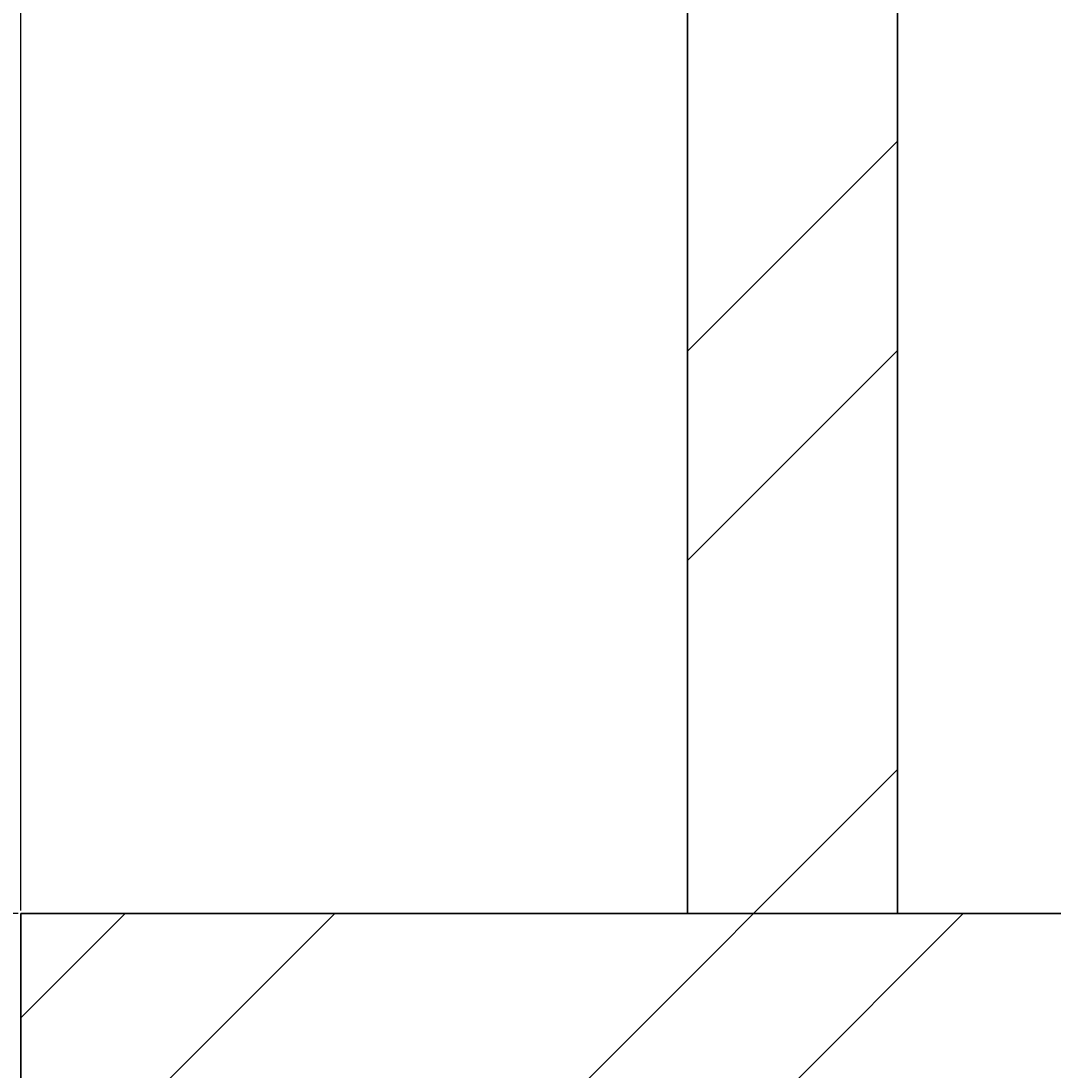
# Model space of a CAD drawing. Units: inches. Extents: x 1962 to 2771, y 1245 to 2660.
# Tile 38 of 114: x 2072.02 to 2094.14, y 2030.47 to 2052.97. Entities that reach past the tile are written whole.
import ezdxf

# ---------------------------------------------------------------- set-up
doc = ezdxf.new("R2010")
doc.units = ezdxf.units.IN
for name, color, linetype, lineweight in [('A-ANNO-DIMS', 2, 'Continuous', 18), ('A-WALL', 7, 'Continuous', 35), ('A-WALL-PATT', 252, 'Continuous', 13)]:
    doc.layers.add(name, color=color, linetype=linetype, lineweight=lineweight)
doc.styles.get("Standard").update_dxf_attribs({"font": 'arial.ttf'})
doc.dimstyles.get("Standard").update_dxf_attribs({"dimtxt": 0.18, "dimasz": 0.18, "dimexe": 0.18, "dimexo": 0.0625, "dimgap": 0.09, "dimtad": 0, "dimtih": 1, "dimtoh": 1, "dimdec": 4, "dimzin": 0, "dimdsep": 46, "dimtxsty": 'Standard', "dimcen": 0.09, "dimadec": 0, "dimazin": 0, "dimtfac": 1, "dimtdec": 4, "dimtofl": 0, "dimtmove": 0, "dimatfit": 3, "dimfxl": 1, "dimtolj": 1, "dimtzin": 0, "dimarcsym": 0})

# ---------------------------------------------------------------- blocks, each defined once
blk = doc.blocks.new('*D40')
at = {"layer": 'A-ANNO-DIMS', "color": 0, "lineweight": -2, "transparency": 16777216}
for p, q in [((2072.02, 2033.906), (2072.02, 2583.474)), ((2660.807, 2524.406), (2660.807, 2583.474)), ((2072.2, 2583.294), (2366.02, 2583.294)), ((2660.627, 2583.294), (2366.808, 2583.294))]:
    blk.add_line(p, q, dxfattribs=at)
at = {"layer": 'A-ANNO-DIMS', "color": 0, "transparency": 16777216}
for points in [[(2072.2, 2583.324), (2072.2, 2583.264), (2072.02, 2583.294)], [(2660.627, 2583.324), (2660.627, 2583.264), (2660.807, 2583.294)]]:
    blk.add_solid(points, dxfattribs=at)
at = {"layer": 'Defpoints', "color": 0, "transparency": 16777216}
for p in [(2660.807, 2583.294), (2660.807, 2524.344), (2072.02, 2033.844)]:
    blk.add_point(p, dxfattribs=at)
at = {"layer": 'A-ANNO-DIMS', "color": 0, "transparency": 16777216, "insert": (2366.414, 2583.294), "char_height": 0.18, "attachment_point": 5}
blk.add_mtext('\\A1;588.8', dxfattribs=at)
blk = doc.blocks.new('*D43')
at = {"layer": 'A-ANNO-DIMS', "color": 0, "lineweight": -2, "transparency": 16777216}
for p, q in [((2086.245, 2524.344), (2012.89, 2524.344)), ((2013.07, 2524.164), (2013.07, 2279.276)), ((2013.07, 2034.024), (2013.07, 2278.912)), ((2071.958, 2033.844), (2012.89, 2033.844))]:
    blk.add_line(p, q, dxfattribs=at)
at = {"layer": 'A-ANNO-DIMS', "color": 0, "transparency": 16777216}
for points in [[(2013.04, 2524.164), (2013.1, 2524.164), (2013.07, 2524.344)], [(2013.04, 2034.024), (2013.1, 2034.024), (2013.07, 2033.844)]]:
    blk.add_solid(points, dxfattribs=at)
at = {"layer": 'Defpoints', "color": 0, "transparency": 16777216}
for p in [(2086.307, 2524.344), (2013.07, 2033.844), (2072.02, 2033.844)]:
    blk.add_point(p, dxfattribs=at)
at = {"layer": 'A-ANNO-DIMS', "color": 0, "transparency": 16777216, "insert": (2013.07, 2279.094), "char_height": 0.18, "attachment_point": 5}
blk.add_mtext('\\A1;490.5', dxfattribs=at)

msp = doc.modelspace()

# ---------------------------------------------------------------- hatches: boundary and pattern name
at = {"layer": 'A-WALL-PATT'}
h = msp.add_hatch(dxfattribs=at)
h.set_pattern_fill('ANSI32', color=256)
h.paths.add_polyline_path([(2090.8074, 2467.3437), (2141.6481, 2467.3437), (2141.6481, 2469.5937), (2141.6481, 2471.8437), (2086.3074, 2471.8437), (2086.3074, 2422.5333), (2090.8074, 2422.5333)])
h.paths.add_polyline_path([(2282.7664, 2471.8437), (2204.8982, 2471.8437), (2204.8982, 2467.3437), (2234.8074, 2467.3437), (2234.8074, 2311.3437), (2228.7492, 2311.3437), (2228.7492, 2306.8437), (2234.8074, 2306.8437), (2331.9227, 2306.8437), (2331.9227, 2309.0937), (2331.9227, 2311.3437), (2239.3074, 2311.3437), (2239.3074, 2467.3437), (2282.7664, 2467.3437), (2282.7664, 2469.5937)])
h.paths.add_polyline_path([(2471.4531, 2519.8437), (2552.011, 2519.8437), (2564.3996, 2519.8437), (2564.3996, 2511.1389), (2568.8996, 2511.1389), (2568.8996, 2524.3437), (2466.9531, 2524.3437), (2466.9531, 2471.8437), (2450.0749, 2471.8437), (2446.4672, 2471.8437), (2446.4672, 2467.3437), (2450.0749, 2467.3437), (2475.9988, 2467.3437), (2475.9988, 2469.5937), (2475.9988, 2471.8437), (2471.4531, 2471.8437)])
h.paths.add_polyline_path([(2575.2231, 2469.5937), (2575.2231, 2471.8437), (2568.8996, 2471.8437), (2568.8996, 2487.1389), (2564.3996, 2487.1389), (2564.3996, 2471.8437), (2556.511, 2471.8437), (2499.2904, 2471.8437), (2499.2904, 2467.3437), (2507.8074, 2467.3437), (2507.8074, 2311.3437), (2414.863, 2311.3437), (2414.863, 2306.8437), (2512.3074, 2306.8437), (2517.0114, 2306.8437), (2517.0114, 2309.0937), (2517.0114, 2311.3437), (2512.3074, 2311.3437), (2512.3074, 2467.3437), (2575.2231, 2467.3437)])
h.paths.add_polyline_path([(2660.8074, 2471.8437), (2600.9602, 2471.8437), (2600.9602, 2467.3437), (2656.3074, 2467.3437), (2656.3074, 2432.5704), (2660.8074, 2432.5704)])
h.paths.add_polyline_path([(2660.8074, 2372.5704), (2656.3074, 2372.5704), (2656.3074, 2311.3437), (2600.276, 2311.3437), (2600.276, 2309.0937), (2600.276, 2306.8437), (2656.3074, 2306.8437), (2656.3074, 2296.2593), (2660.8074, 2296.2593)])
h.paths.add_polyline_path([(2572.3074, 2306.8437), (2577.1385, 2306.8437), (2577.1385, 2311.3437), (2551.082, 2311.3437), (2551.082, 2306.8437), (2567.8074, 2306.8437), (2567.8074, 2258.8437), (2540.0574, 2258.8437), (2540.0574, 2256.5937), (2540.0574, 2254.3437), (2567.8074, 2254.3437), (2656.3074, 2254.3437), (2656.3074, 2236.9085), (2660.8074, 2236.9085), (2660.8074, 2272.2593), (2656.3074, 2272.2593), (2656.3074, 2258.8437), (2572.3074, 2258.8437)])
h.paths.add_polyline_path([(2512.3074, 2254.3437), (2518.8716, 2254.3437), (2518.8716, 2256.5937), (2518.8716, 2258.8437), (2507.8074, 2258.8437), (2507.8074, 2177.8437), (2567.8074, 2177.8437), (2567.8074, 2172.9628), (2572.3074, 2172.9628), (2572.3074, 2177.8437), (2656.3074, 2177.8437), (2656.3074, 2166.4846), (2660.8074, 2166.4846), (2660.8074, 2200.9085), (2656.3074, 2200.9085), (2656.3074, 2182.3437), (2512.3074, 2182.3437)])
h.paths.add_polyline_path([(2656.3074, 2129.8437), (2572.3074, 2129.8437), (2572.3074, 2150.3044), (2570.0574, 2150.3044), (2567.8074, 2150.3044), (2567.8074, 2129.8437), (2507.8074, 2129.8437), (2507.8074, 2116.3027), (2510.0574, 2116.3027), (2512.3074, 2116.3027), (2512.3074, 2125.3437), (2567.8074, 2125.3437), (2572.3074, 2125.3437), (2656.3074, 2125.3437)])
h.paths.add_polyline_path([(2090.8074, 2362.5333), (2086.3074, 2362.5333), (2086.3074, 2298.6242), (2090.8074, 2298.6242), (2090.8074, 2306.8437), (2174.8074, 2306.8437), (2174.8074, 2286.4178), (2179.3074, 2286.4178), (2179.3074, 2306.8437), (2192.8641, 2306.8437), (2192.8641, 2309.0937), (2192.8641, 2311.3437), (2090.8074, 2311.3437)])
h.paths.add_polyline_path([(2209.156, 2258.8437), (2179.3074, 2258.8437), (2179.3074, 2263.2236), (2177.0574, 2263.2236), (2174.8074, 2263.2236), (2174.8074, 2258.8437), (2090.8074, 2258.8437), (2090.8074, 2274.6242), (2086.3074, 2274.6242), (2086.3074, 2238.2967), (2088.5574, 2238.2967), (2090.8074, 2238.2967), (2090.8074, 2254.3437), (2209.156, 2254.3437)])
h.paths.add_polyline_path([(2090.8074, 2177.8437), (2234.8074, 2177.8437), (2234.8074, 2173.1428), (2239.3074, 2173.1428), (2239.3074, 2258.8437), (2230.8442, 2258.8437), (2230.8442, 2256.5937), (2230.8442, 2254.3437), (2234.8074, 2254.3437), (2234.8074, 2182.3437), (2090.8074, 2182.3437), (2090.8074, 2202.2967), (2086.3074, 2202.2967), (2086.3074, 2140.0389), (2090.8074, 2140.0389)])
h.paths.add_polyline_path([(2090.8074, 2080.0389), (2086.3074, 2080.0389), (2086.3074, 2033.8437), (2090.8074, 2033.8437)], flags=17)
h.paths.add_polyline_path([(2244.9405, 2033.8437), (2239.3074, 2033.8437), (2239.3074, 2142.0665), (2237.2592, 2142.0665), (2234.8074, 2142.0665), (2234.8074, 2033.8437), (2090.8074, 2033.8437), (2076.5204, 2033.8437), (2072.0204, 2033.8437), (2072.0204, 2000.4493), (2076.5204, 2000.4493), (2076.5204, 2029.3437), (2090.8074, 2029.3437), (2244.9405, 2029.3437), (2244.9405, 2031.5937)])
h.paths.add_polyline_path([(2234.8074, 1933.3437), (2076.5204, 1933.3437), (2076.5204, 1952.4493), (2074.2704, 1952.4493), (2072.0204, 1952.4493), (2072.0204, 1933.3437), (2072.0204, 1928.8437), (2234.8074, 1928.8437)])
h.paths.add_polyline_path([(2090.8074, 1928.8437), (2086.3074, 1928.8437), (2086.3074, 1906.5013), (2090.8074, 1906.5013)])
h.paths.add_polyline_path([(2090.8074, 1846.5013), (2086.3074, 1846.5013), (2086.3074, 1769.9917), (2088.5574, 1769.9917), (2090.8074, 1769.9917), (2090.8074, 1780.3437), (2234.8074, 1780.3437), (2234.8074, 1708.3437), (2230.3764, 1708.3437), (2230.3764, 1703.8437), (2239.3074, 1703.8437), (2239.3074, 1792.6669), (2237.0574, 1792.6669), (2234.8074, 1792.6669), (2234.8074, 1784.8437), (2090.8074, 1784.8437)])
h.paths.add_polyline_path([(2239.3074, 1928.8437), (2244.9405, 1928.8437), (2244.9405, 1931.0937), (2244.9405, 1933.3437), (2234.8074, 1933.3437), (2234.8074, 1928.8437), (2234.8074, 1825.5949), (2239.3074, 1825.5949)])
h.paths.add_polyline_path([(2148.0425, 1649.0937), (2148.0425, 1651.3437), (2090.8074, 1651.3437), (2090.8074, 1646.8437), (2148.0425, 1646.8437)], flags=0)
h.paths.add_polyline_path([(2207.5601, 1708.3437), (2090.8074, 1708.3437), (2090.8074, 1703.8437), (2174.8074, 1703.8437), (2174.8074, 1651.3437), (2170.4457, 1651.3437), (2170.4457, 1646.8437), (2195.9924, 1646.8437), (2195.9924, 1649.0937), (2195.9924, 1651.3437), (2179.3074, 1651.3437), (2179.3074, 1703.8437), (2207.5601, 1703.8437), (2207.5601, 1706.0937)])
h.paths.add_polyline_path([(2090.8074, 1733.9917), (2086.3074, 1733.9917), (2086.3074, 1696.1032), (2088.5574, 1696.1032), (2090.8074, 1696.1032)])
h.paths.add_polyline_path([(2090.8074, 1672.1032), (2086.3074, 1672.1032), (2086.3074, 1600.3335), (2090.8074, 1600.3335)])
h.paths.add_polyline_path([(2090.8074, 1540.3335), (2086.3074, 1540.3335), (2086.3074, 1486.3437), (2139.6766, 1486.3437), (2139.6766, 1490.8437), (2090.8074, 1490.8437)])
h.paths.add_polyline_path([(2302.3876, 1490.8437), (2239.3074, 1490.8437), (2239.3074, 1646.8437), (2335.9994, 1646.8437), (2335.9994, 1651.3437), (2229.884, 1651.3437), (2229.884, 1646.8437), (2234.8074, 1646.8437), (2234.8074, 1490.8437), (2202.7103, 1490.8437), (2202.7103, 1488.5937), (2202.7103, 1486.3437), (2275.0699, 1486.3437), (2275.0699, 1475.772), (2279.5699, 1475.772), (2279.5699, 1486.3437), (2302.3876, 1486.3437)])
h.paths.add_polyline_path([(2279.5699, 1451.772), (2275.0699, 1451.772), (2275.0699, 1438.3437), (2174.8074, 1438.3437), (2174.8074, 1486.3437), (2179.7922, 1486.3437), (2179.7922, 1490.8437), (2163.3585, 1490.8437), (2163.3585, 1488.5937), (2163.3585, 1486.3437), (2170.3074, 1486.3437), (2170.3074, 1433.8437), (2279.5699, 1433.8437)])
h.paths.add_polyline_path([(2427.2363, 1490.8437), (2375.8074, 1490.8437), (2375.8074, 1646.8437), (2381.6401, 1646.8437), (2381.6401, 1651.3437), (2365.887, 1651.3437), (2365.887, 1649.0937), (2365.887, 1646.8437), (2371.3074, 1646.8437), (2371.3074, 1490.8437), (2327.5627, 1490.8437), (2327.5627, 1488.5937), (2327.5627, 1486.3437), (2371.3074, 1486.3437), (2371.3074, 1433.8437), (2375.8074, 1433.8437), (2375.8074, 1486.3437), (2427.2363, 1486.3437)])
h.paths.add_polyline_path([(2512.3074, 1646.8437), (2519.4351, 1646.8437), (2519.4351, 1649.0937), (2519.4351, 1651.3437), (2507.8074, 1651.3437), (2416.0063, 1651.3437), (2416.0063, 1649.0937), (2416.0063, 1646.8437), (2507.8074, 1646.8437), (2507.8074, 1490.8437), (2497.0532, 1490.8437), (2497.0532, 1488.5937), (2497.0532, 1486.3437), (2574.9344, 1486.3437), (2574.9344, 1476.0181), (2579.4344, 1476.0181), (2579.4344, 1486.3437), (2584.4872, 1486.3437), (2584.3074, 1490.8437), (2512.3074, 1490.8437)])
h.paths.add_polyline_path([(2470.5091, 1486.3437), (2473.9767, 1486.3437), (2473.9767, 1490.8437), (2449.6605, 1490.8437), (2449.6605, 1488.5937), (2449.6605, 1486.3437), (2466.0091, 1486.3437), (2466.0091, 1433.8437), (2470.5091, 1433.8437), (2579.4344, 1433.8437), (2579.4344, 1452.0181), (2574.9344, 1452.0181), (2574.9344, 1438.3437), (2554.5091, 1438.3437), (2470.5091, 1438.3437)])
h.paths.add_polyline_path([(2656.3074, 1490.8437), (2611.86, 1490.8437), (2611.86, 1486.3437), (2656.3074, 1486.3437)])
h.paths.add_polyline_path([(2660.8074, 1532.7007), (2658.5574, 1532.7007), (2656.3074, 1532.7007), (2656.3074, 1486.3437), (2660.8074, 1486.3437)])
h.paths.add_polyline_path([(2660.8074, 1664.9663), (2656.3074, 1664.9663), (2656.3074, 1651.3437), (2602.2313, 1651.3437), (2602.2313, 1646.8437), (2656.3074, 1646.8437), (2656.3074, 1592.7007), (2660.8074, 1592.7007)])
h.paths.add_polyline_path([(2660.8074, 1724.5221), (2656.3074, 1724.5221), (2656.3074, 1703.8437), (2542.4725, 1703.8437), (2542.4725, 1699.3437), (2567.8074, 1699.3437), (2567.8074, 1651.3437), (2552.7766, 1651.3437), (2552.7766, 1649.0937), (2552.7766, 1646.8437), (2577.2878, 1646.8437), (2577.2878, 1649.0937), (2577.2878, 1651.3437), (2572.3074, 1651.3437), (2572.3074, 1699.3437), (2656.3074, 1699.3437), (2656.3074, 1688.9663), (2660.8074, 1688.9663)])
h.paths.add_polyline_path([(2660.8074, 1880.6524), (2656.3074, 1880.6524), (2656.3074, 1832.8437), (2512.3074, 1832.8437), (2512.3074, 1837.8959), (2507.8074, 1837.8959), (2507.8074, 1828.3437), (2567.8074, 1828.3437), (2567.8074, 1804.3437), (2572.3074, 1804.3437), (2572.3074, 1828.3437), (2656.3074, 1828.3437), (2656.3074, 1818.6778), (2660.8074, 1818.6778)])
h.paths.add_polyline_path([(2660.8074, 1794.6778), (2656.3074, 1794.6778), (2656.3074, 1780.3437), (2572.3074, 1780.3437), (2572.3074, 1783.0303), (2570.0574, 1783.0303), (2567.8074, 1783.0303), (2567.8074, 1780.3437), (2507.8074, 1780.3437), (2507.8074, 1699.3437), (2517.8858, 1699.3437), (2517.8858, 1701.5937), (2517.8858, 1703.8437), (2512.3074, 1703.8437), (2512.3074, 1775.8437), (2656.3074, 1775.8437), (2656.3074, 1760.5221), (2660.8074, 1760.5221)])
h.paths.add_polyline_path([(2660.8074, 1981.3437), (2660.8074, 2020.2808), (2658.5574, 2020.2808), (2656.3074, 2020.2808), (2656.3074, 1981.3437), (2512.3074, 1981.3437), (2512.3074, 2086.6996), (2507.8074, 2086.6996), (2507.8074, 1981.3437), (2375.8074, 1981.3437), (2375.8074, 1986.8505), (2373.5574, 1986.8505), (2371.3074, 1986.8505), (2371.3074, 1973.2607), (2375.8074, 1973.2607), (2375.8074, 1976.8437), (2507.8074, 1976.8437), (2507.8074, 1865.4281), (2510.0574, 1865.4281), (2512.3074, 1865.4281), (2512.3074, 1976.8437), (2660.8074, 1976.8437)])
h.paths.add_polyline_path([(2375.8074, 1940.297), (2373.5574, 1940.297), (2371.3074, 1940.297), (2371.3074, 1933.3437), (2278.4434, 1933.3437), (2278.4434, 1928.8437), (2371.3074, 1928.8437), (2371.3074, 1651.3437), (2375.8074, 1651.3437)])
h.paths.add_polyline_path([(2660.8074, 1976.8437), (2656.3074, 1976.8437), (2656.3074, 1940.6524), (2660.8074, 1940.6524)], flags=17)
h.paths.add_polyline_path([(2660.8074, 2142.4846), (2656.3074, 2142.4846), (2656.3074, 2080.2808), (2660.8074, 2080.2808)])
h.paths.add_polyline_path([(2381.4189, 2311.3437), (2375.8074, 2311.3437), (2375.8074, 2467.3437), (2424.7242, 2467.3437), (2424.7242, 2469.5937), (2424.7242, 2471.8437), (2375.8074, 2471.8437), (2375.8074, 2524.3437), (2371.3074, 2524.3437), (2371.3074, 2471.8437), (2307.2097, 2471.8437), (2307.2097, 2467.3437), (2371.3074, 2467.3437), (2371.3074, 2311.3437), (2366.8901, 2311.3437), (2366.8901, 2306.8437), (2371.3074, 2306.8437), (2371.3074, 2033.8437), (2279.6589, 2033.8437), (2279.6589, 2029.3437), (2371.3074, 2029.3437), (2371.3074, 2014.2598), (2375.8074, 2014.2598), (2375.8074, 2306.8437), (2381.4189, 2306.8437)])
h.paths.add_polyline_path([(2263.3074, 2524.3437), (2170.3074, 2524.3437), (2170.3074, 2519.8437), (2170.3074, 2471.8437), (2165.0312, 2471.8437), (2165.0312, 2467.3437), (2179.6721, 2467.3437), (2179.6721, 2469.5161), (2179.6721, 2471.8437), (2174.8074, 2471.8437), (2174.8074, 2519.8437), (2258.8074, 2519.8437), (2258.8074, 2511.6436), (2263.3074, 2511.6436)])
h.paths.add_polyline_path([(2245.0232, 1361.4123), (2492.9468, 1361.4123), (2492.9468, 1398.505), (2245.0232, 1398.505)], flags=9)
h.paths.add_polyline_path([(2388.1434, 2086.6936), (2425.0704, 2086.6936), (2425.0704, 2105.3509), (2388.1434, 2105.3509)], flags=9)
h.paths.add_polyline_path([(2404.922, 2242.6744), (2445.7337, 2242.6744), (2445.7337, 2261.3318), (2404.922, 2261.3318)], flags=9)
h.paths.add_polyline_path([(2269.4107, 2156.7935), (2306.3378, 2156.7935), (2306.3378, 2175.4508), (2269.4107, 2175.4508)], flags=9)
h.paths.add_polyline_path([(2269.3277, 2233.4343), (2306.2547, 2233.4343), (2306.2547, 2252.0917), (2269.3277, 2252.0917)], flags=9)
h.paths.add_polyline_path([(2431.6052, 2320.6922), (2470.4456, 2320.6922), (2470.4456, 2339.3495), (2431.6052, 2339.3495)], flags=25)
h.paths.add_polyline_path([(2249.6902, 2315.7608), (2288.5306, 2315.7608), (2288.5306, 2334.4182), (2249.6902, 2334.4182)], flags=25)
h.paths.add_polyline_path([(2096.9301, 2314.3181), (2135.7704, 2314.3181), (2135.7704, 2332.9755), (2096.9301, 2332.9755)], flags=25)
h.paths.add_polyline_path([(2134.3475, 2285.7089), (2161.4655, 2285.7089), (2161.4655, 2304.3662), (2134.3475, 2304.3662)], flags=9)
h.paths.add_polyline_path([(2126.5155, 2209.4076), (2159.9227, 2209.4076), (2159.9227, 2228.065), (2126.5155, 2228.065)], flags=25)
h.paths.add_polyline_path([(2110.5753, 2141.5299), (2149.4157, 2141.5299), (2149.4157, 2160.1872), (2110.5753, 2160.1872)], flags=25)
h.paths.add_polyline_path([(2249.8618, 1968.3317), (2286.3966, 1968.3317), (2286.3966, 1986.989), (2249.8618, 1986.989)], flags=9)
h.paths.add_polyline_path([(2395.9507, 1777.0051), (2436.7624, 1777.0051), (2436.7624, 1795.6625), (2395.9507, 1795.6625)], flags=9)
h.paths.add_polyline_path([(2398.5259, 1888.5651), (2435.0062, 1888.5651), (2435.0062, 1907.2224), (2398.5259, 1907.2224)], flags=25)
h.paths.add_polyline_path([(2259.3506, 1728.3559), (2296.2776, 1728.3559), (2296.2776, 1747.0132), (2259.3506, 1747.0132)], flags=9)
h.paths.add_polyline_path([(2271.3698, 1845.268), (2308.2968, 1845.268), (2308.2968, 1863.9253), (2271.3698, 1863.9253)], flags=9)
h.paths.add_polyline_path([(2120.9355, 1786.3027), (2159.7759, 1786.3027), (2159.7759, 1804.9601), (2120.9355, 1804.9601)], flags=25)
h.paths.add_polyline_path([(2121.3164, 1732.1043), (2154.7236, 1732.1043), (2154.7236, 1750.7616), (2121.3164, 1750.7616)], flags=25)
h.paths.add_polyline_path([(2118.3706, 1678.8997), (2147.5282, 1678.8997), (2147.5282, 1697.557), (2118.3706, 1697.557)], flags=25)
h.paths.add_polyline_path([(2385.9227, 1493.557), (2424.763, 1493.557), (2424.763, 1512.2143), (2385.9227, 1512.2143)], flags=25)
h.paths.add_polyline_path([(2248.7058, 1500.0256), (2287.5462, 1500.0256), (2287.5462, 1518.6829), (2248.7058, 1518.6829)], flags=25)
h.paths.add_polyline_path([(2104.1669, 1617.3771), (2143.0073, 1617.3771), (2143.0073, 1636.0344), (2104.1669, 1636.0344)], flags=9)
h.paths.add_polyline_path([(2096.0714, 1447.8824), (2137.3845, 1447.8824), (2137.3845, 1458.1859), (2096.0714, 1458.1859)], flags=9)
h.paths.add_polyline_path([(2180.6114, 1440.325), (2209.7689, 1440.325), (2209.7689, 1458.9823), (2180.6114, 1458.9823)], flags=25)
h.paths.add_polyline_path([(2316.1698, 1447.9637), (2357.4829, 1447.9637), (2357.4829, 1458.2673), (2316.1698, 1458.2673)], flags=9)
h.paths.add_polyline_path([(2397.6187, 1447.9637), (2438.9318, 1447.9637), (2438.9318, 1458.2673), (2397.6187, 1458.2673)], flags=9)
h.paths.add_polyline_path([(2473.0778, 1439.5953), (2502.2354, 1439.5953), (2502.2354, 1458.2527), (2473.0778, 1458.2527)], flags=25)
h.paths.add_polyline_path([(2589.7027, 1447.8819), (2631.0158, 1447.8819), (2631.0158, 1458.1855), (2589.7027, 1458.1855)], flags=9)
h.paths.add_polyline_path([(2522.4009, 1497.5285), (2561.2413, 1497.5285), (2561.2413, 1516.1859), (2522.4009, 1516.1859)], flags=25)
h.paths.add_polyline_path([(2579.6565, 1671.3482), (2608.8141, 1671.3482), (2608.8141, 1690.0056), (2579.6565, 1690.0056)], flags=25)
h.paths.add_polyline_path([(2544.7038, 1725.5064), (2578.1111, 1725.5064), (2578.1111, 1744.1637), (2544.7038, 1744.1637)], flags=25)
h.paths.add_polyline_path([(2578.1191, 1807.472), (2607.2766, 1807.472), (2607.2766, 1826.1293), (2578.1191, 1826.1293)], flags=25)
h.paths.add_polyline_path([(2595.0614, 1835.1839), (2633.9018, 1835.1839), (2633.9018, 1853.8413), (2595.0614, 1853.8413)], flags=25)
h.paths.add_polyline_path([(2567.0097, 2097.7035), (2605.8501, 2097.7035), (2605.8501, 2116.3609), (2567.0097, 2116.3609)], flags=9)
h.paths.add_polyline_path([(2586.644, 2134.6454), (2615.8015, 2134.6454), (2615.8015, 2153.3027), (2586.644, 2153.3027)], flags=9)
h.paths.add_polyline_path([(2544.6185, 2212.6783), (2578.0258, 2212.6783), (2578.0258, 2231.3356), (2544.6185, 2231.3356)], flags=25)
h.paths.add_polyline_path([(2577.0273, 2256.9023), (2606.1849, 2256.9023), (2606.1849, 2275.5597), (2577.0273, 2275.5597)], flags=24)
h.paths.add_polyline_path([(2605.2683, 2315.2821), (2644.1087, 2315.2821), (2644.1087, 2333.9395), (2605.2683, 2333.9395)], flags=25)
h.paths.add_polyline_path([(2583.1244, 2496.1815), (2624.4375, 2496.1815), (2624.4375, 2506.4851), (2583.1244, 2506.4851)], flags=9)
h.paths.add_polyline_path([(2474.761, 2497.0823), (2503.9185, 2497.0823), (2503.9185, 2515.7397), (2474.761, 2515.7397)], flags=25)
h.paths.add_polyline_path([(2387.5787, 2494.2563), (2428.902, 2494.2563), (2428.902, 2504.5598), (2387.5787, 2504.5598)], flags=9)
h.paths.add_polyline_path([(2300.1657, 2500.1564), (2341.4788, 2500.1564), (2341.4788, 2510.46), (2300.1657, 2510.46)], flags=25)
h.paths.add_polyline_path([(2176.8589, 2497.5843), (2206.0165, 2497.5843), (2206.0165, 2516.2416), (2176.8589, 2516.2416)], flags=25)
h.paths.add_polyline_path([(2097.4668, 2494.9762), (2138.7799, 2494.9762), (2138.7799, 2505.2798), (2097.4668, 2505.2798)], flags=9)

# ---------------------------------------------------------------- linework, layer by layer
at = {"layer": 'A-WALL'}
for p, q in [((2086.3074, 2471.8437), (2086.3074, 2033.8437)), ((2090.8074, 2177.8437), (2090.8074, 2033.8437)), ((2076.5204, 2033.8437), (2072.0204, 2033.8437)), ((2072.0204, 2033.8437), (2072.0204, 1933.3437)), ((2090.8074, 2033.8437), (2076.5204, 2033.8437)), ((2090.8074, 2033.8437), (2234.8074, 2033.8437))]:
    msp.add_line(p, q, dxfattribs=at)

# ---------------------------------------------------------------- dimensions: what is measured, and where the dimension line sits
at = {"layer": 'A-ANNO-DIMS'}
dim = msp.add_linear_dim(base=(2660.8074, 2583.2937), p1=(2072.0204, 2033.8437), p2=(2660.8074, 2524.3437), dimstyle='Standard', override={"dimdec": 1, "dimlfac": 1, "dimrnd": 0, "dimzin": 0, "dimdsep": 46, "dimlunit": 2}, dxfattribs=at)
dim.commit()
dim.dimension.update_dxf_attribs({"geometry": '*D40', "text_midpoint": (2366.4139, 2583.2937)})
dim = msp.add_linear_dim(base=(2013.0704, 2033.8437), p1=(2086.3074, 2524.3437), p2=(2072.0204, 2033.8437), angle=90, dimstyle='Standard', override={"dimdec": 1, "dimlfac": 1, "dimrnd": 0, "dimzin": 0, "dimdsep": 46, "dimlunit": 2}, dxfattribs=at)
dim.commit()
dim.dimension.update_dxf_attribs({"geometry": '*D43', "text_midpoint": (2013.0704, 2279.0937)})

doc.saveas('drawing.dxf')
